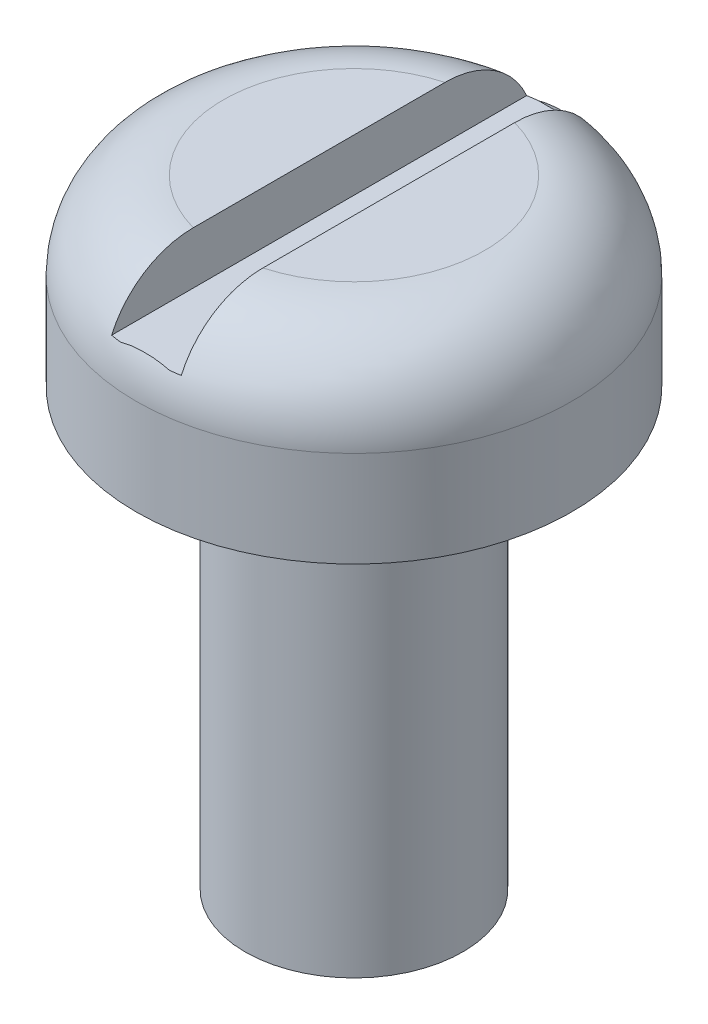
SolidWorks part; units mm, degrees
material "Plain Carbon Steel"
ref_plane "Front Plane" through (0, 0, 0) normal (0, 0, 1) x (1, 0, 0)
ref_plane "Top Plane" through (0, 0, 0) normal (0, 1, 0) x (1, 0, 0)
ref_plane "Right Plane" through (0, 0, 0) normal (1, 0, 0) x (0, 0, -1)
sketch "Bolt Profile Sketch" plane through (0, 0, 0) normal (0, 0, 1) x (1, 0, 0)
  line L0 (0, 4.111) -> (0, -3.1618) construction
  line L1 (0, -5) -> (1.25, -5)
  line L2 (1.25, -5) -> (1.25, 0)
  line L3 (1.25, 0) -> (2.5, 0)
  line L4 (2.5, 0) -> (2.5, 2.1)
  line L6 (0, 2.1) -> (0, -5)
  line L7 (0, 2.1) -> (2.5, 2.1)
  dimension "D4" = 7.1
  dimension "D1" = 1.25
  dimension "D2" = 2.5
  dimension "D3" = 2.1
revolve "Bolt Body Ø2.5 Shank Ø5 Head" add sketch "Bolt Profile Sketch" angle 360 about L0
fillet "Head Edge Fillet R1" radius 1 1 edges at (0, 2.1, 2.5)
sketch "Screwdriver Slot Sketch" plane through (0, 2.1, 0) normal (0, 1, 0) x (1, 0, 0)
  line L1 (-0.4, -2.4) -> (0.4, -2.4)
  line L2 (-0.4, -2.4) -> (-0.4, 2.4)
  line L3 (-0.4, 2.4) -> (0.4, 2.4)
  line L4 (0.4, -2.4) -> (0.4, 2.4)
  line L5 (-0.4, -2.4) -> (0.4, 2.4) construction
  line L6 (-0.4, 2.4) -> (0.4, -2.4) construction
  point P0 (0, 0)
  dimension "D1" = 0.8
  dimension "D2" = 4.8
extrude "Screwdriver Slot 0.8 x 0.6" cut sketch "Screwdriver Slot Sketch" against normal blind 0.6
